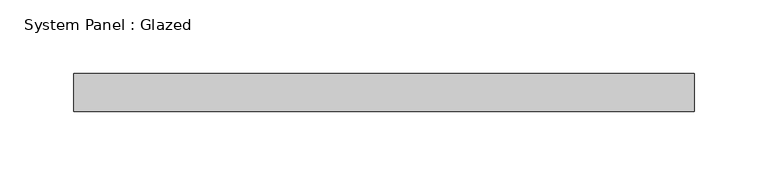
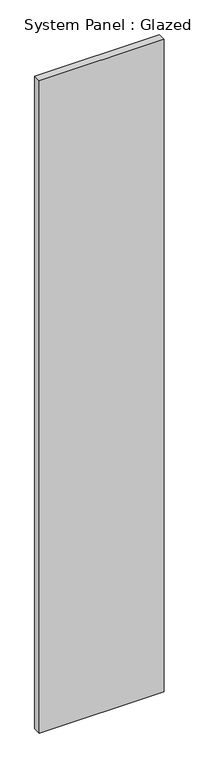
"""IFC4 building model written with IfcOpenShell, lengths in millimetres: plate geometry, System Panel : Glazed."""

from ifc_helpers import new_model, si_unit, origin, origin_with_axes, place, context, project, spatial, polyline, outline, extrude, source, transform, mapped, element, save


def system_panel_glazed_1f7552f7(model_context):
    return source(origin(), model_context, "Body", "SweptSolid", [
        extrude(outline(polyline([(209.5334635, 19.05), (-209.5334635, 19.05), (-209.5334635, 44.45), (209.5334635, 44.45), (209.5334635, 19.05)])), origin_with_axes(), (0.0, 0.0, 1.0), 2311.4),
    ])


if __name__ == "__main__":
    model = new_model("IFC4")
    model_context = context("Model", 3, world=origin())
    ifc_project = project(units=[si_unit("LENGTHUNIT", "METRE", prefix="MILLI")], contexts=[model_context])
    site = spatial("IfcSite", under=ifc_project)
    building = spatial("IfcBuilding", under=site)
    placement = place(None, origin())
    system_panel_glazed_shape = system_panel_glazed_1f7552f7(model_context)
    element("IfcPlate", 1, ObjectType="System Panel : Glazed", at=placement, inside=building, context=model_context, shape_type="MappedRepresentation", body=[
        mapped(system_panel_glazed_shape, transform((0.0, 0.0, 0.0), x_axis=(1.0, 0.0, 0.0), y_axis=(0.0, 1.0, 0.0), z_axis=(0.0, 0.0, 1.0))),
    ])
    save(model, "model.ifc")

# Revit data of these elements
# Type "System Panel : Glazed"
#   Construction Type Id = "GSP4R"
#   Analytic Construction = "1/8 in Pilkington single glazing"
#   Visual Light Transmittance = 0.9
#   Solar Heat Gain Coefficient = 0.86
#   Heat Transfer Coefficient (U) = 1.18115 BTU/(h·ft²·°F)
#   Define Thermal Properties by = 1
# Element 1 (IfcPlate, "System Panel : Glazed")
#   Materials on its faces: "Glass"
# Materials
#   "Glass": class "Glass", colour RGB 0 128 192, transparency 0.75, Description = "Soda Lime Glass", Cost = 0
